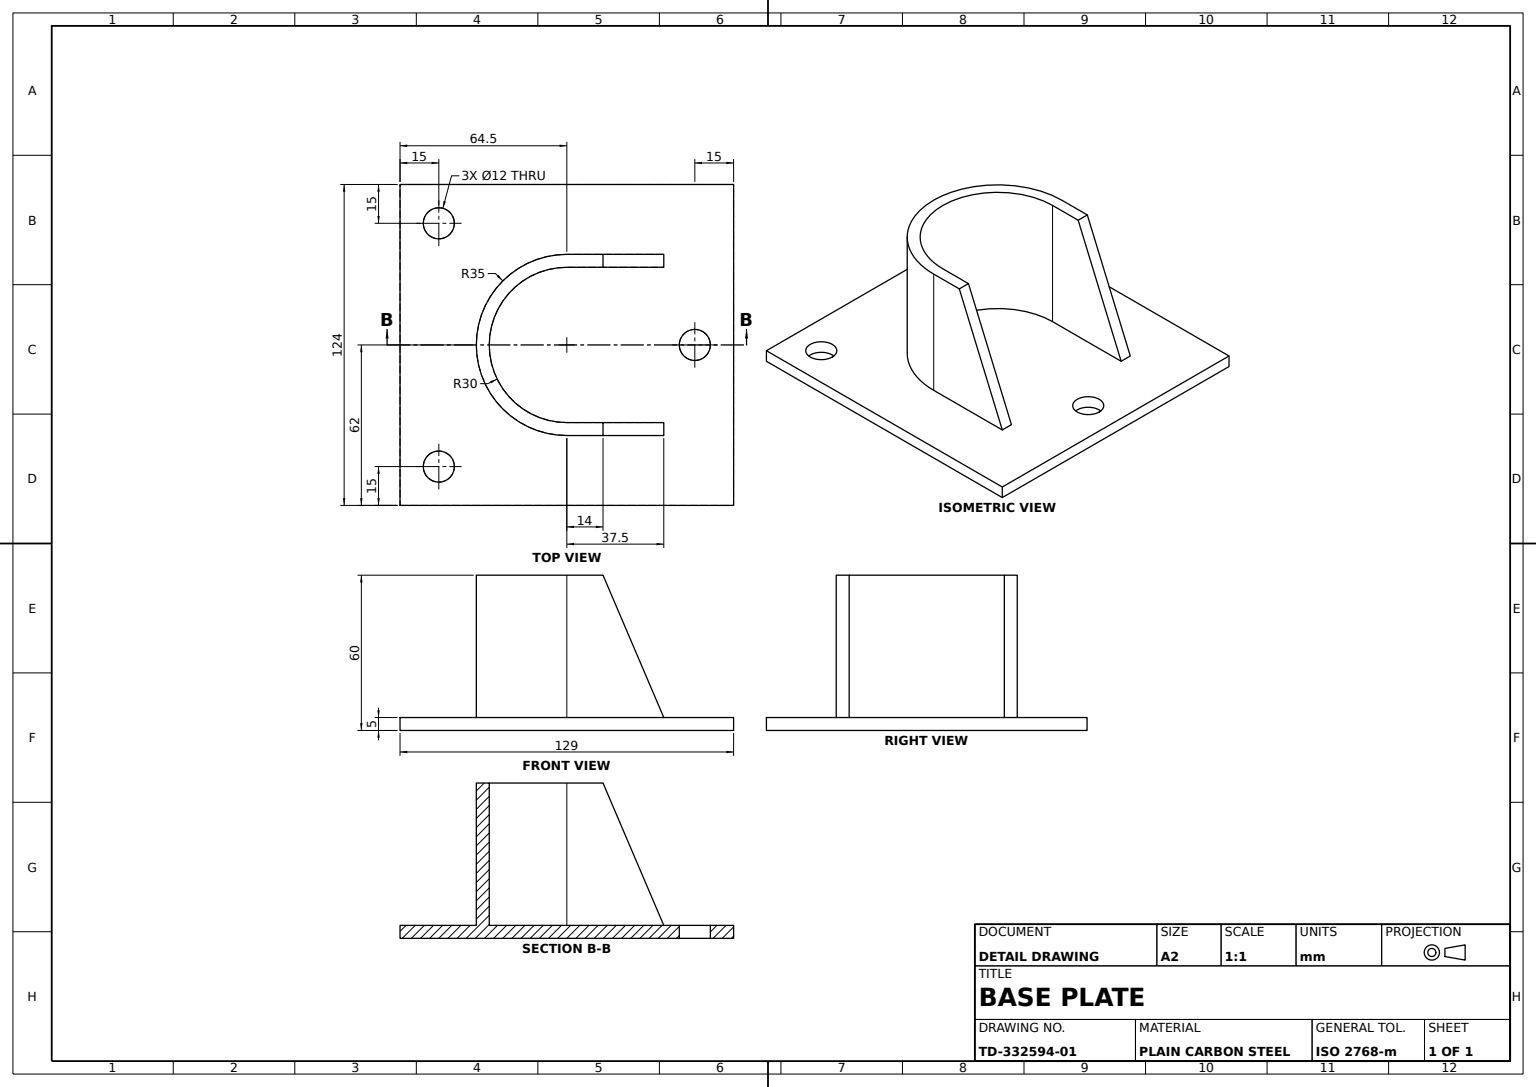
from build123d import *

# Parameters (mm, degrees)
BASE_PLATE_SKETCH_W         = 124
BASE_PLATE_SKETCH_H         = 129
BASE_PLATE_SKETCH_R         = 6
BASE_PLATE_DEPTH            = 5
UPRIGHT_SUPPORT_BLOCK_DEPTH = 35
CRADLE_CUT_SKETCH_W         = 60
CRADLE_CUT_SKETCH_H         = 23.5
CRADLE_CUT_DEPTH            = 55
GUSSET_TRIM_CUT_DEPTH       = 55


with BuildPart() as part:
    # Base Plate Sketch → Base Plate (new body)
    with BuildSketch(Plane(origin=(0, 0, 0), x_dir=(1, 0, 0), z_dir=(0, 1, 0))):
        Rectangle(BASE_PLATE_SKETCH_W, BASE_PLATE_SKETCH_H)
        with Locations(Location((0, 49.5, 0), (0, 0, 270))):
            Circle(BASE_PLATE_SKETCH_R, mode=Mode.SUBTRACT)
        with Locations(Location((47, -49.5, 0), (0, 0, 270))):
            Circle(BASE_PLATE_SKETCH_R, mode=Mode.SUBTRACT)
        with Locations(Location((-47, -49.5, 0), (0, 0, 270))):
            Circle(BASE_PLATE_SKETCH_R, mode=Mode.SUBTRACT)
    extrude(amount=BASE_PLATE_DEPTH)

    # Upright Support Profile Sketch → Upright Support Block (add, symmetric)
    with BuildSketch(Plane(origin=(0, 0, 0), x_dir=(0, 0, -1), z_dir=(1, 0, 0))):
        Polygon((37.5, 5), (14, 60), (-35, 60), (-35, 5), align=None)
    extrude(amount=UPRIGHT_SUPPORT_BLOCK_DEPTH, both=True)

    # Cradle Cut Sketch → Cradle Cut (cut)
    with BuildSketch(Plane(origin=(0, 60, 0), x_dir=(1, 0, 0), z_dir=(0, 1, 0))):
        with Locations((0, 25.75)):
            Rectangle(CRADLE_CUT_SKETCH_W, CRADLE_CUT_SKETCH_H)
        with BuildLine():
            Line((30, 14), (-30, 14))
            Line((-30, 14), (-30, 0))
            ThreePointArc((-30, 0), (0, -30), (30, 0))
            Line((30, 0), (30, 14))
        make_face()
    extrude(amount=-CRADLE_CUT_DEPTH, mode=Mode.SUBTRACT)

    # Gusset Trim Sketch → Gusset Trim Cut (cut)
    with BuildSketch(Plane(origin=(0, 60, 0), x_dir=(1, 0, 0), z_dir=(0, 1, 0))):
        with BuildLine():
            Line((-35, -35), (1.7e-07, -35))
            ThreePointArc((1.7e-07, -35), (-24.748737282, -24.748737402), (-35, 0))
            Line((-35, 0), (-35, -35))
        make_face()
        with BuildLine():
            Line((35, -35), (35, 0))
            ThreePointArc((35, 0), (24.748737402, -24.748737282), (1.7e-07, -35))
            Line((1.7e-07, -35), (35, -35))
        make_face()
    extrude(amount=-GUSSET_TRIM_CUT_DEPTH, mode=Mode.SUBTRACT)


solid = part.part
